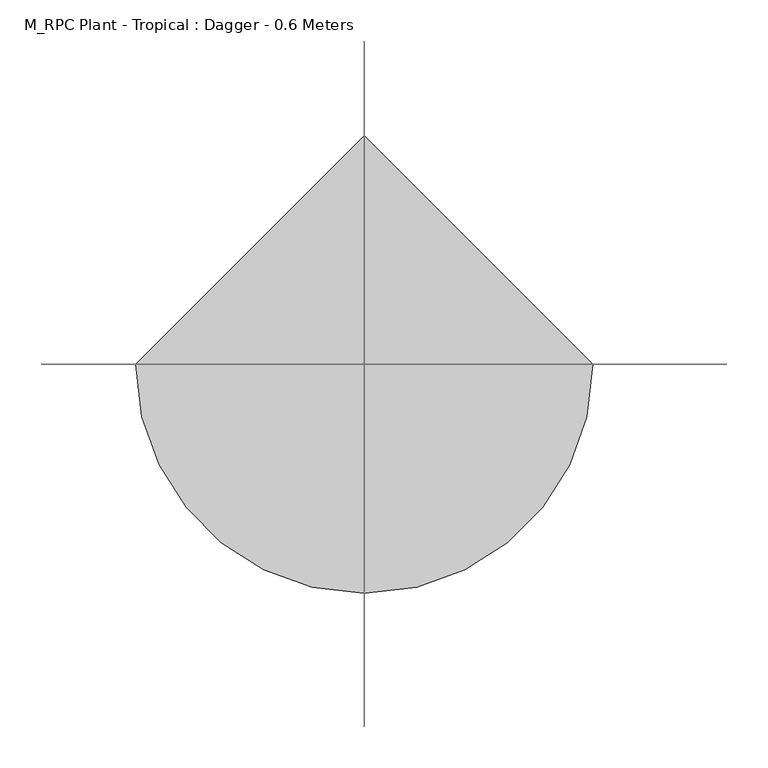
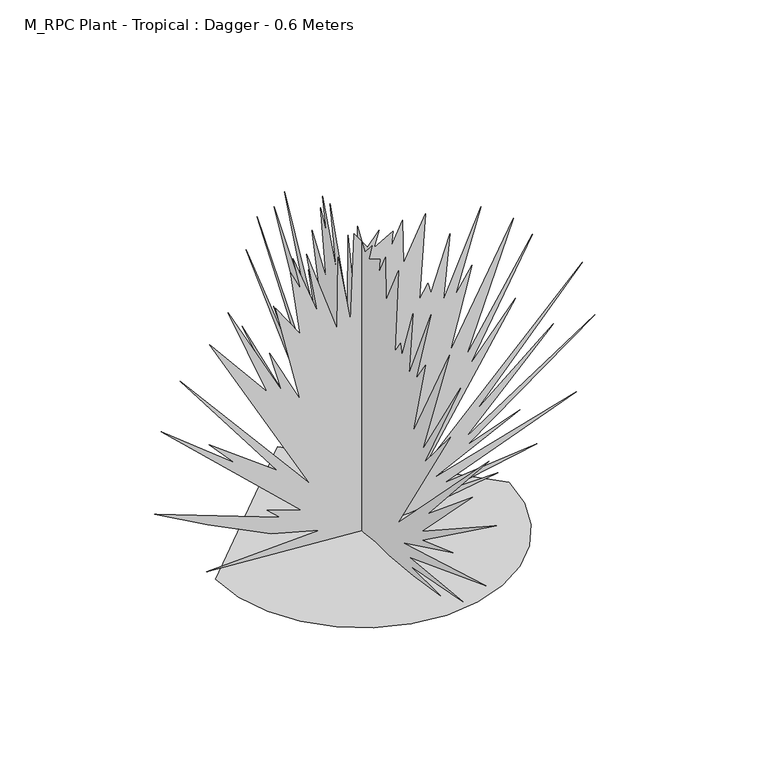
"""IFC4 building model written with IfcOpenShell, lengths in millimetres: geographic element geometry, M_RPC Plant - Tropical : Dagger - 0.6 Meters."""

from ifc_helpers import new_model, si_unit, origin, place, context, project, spatial, triangles, source, transform, mapped, element, save


def m_rpc_plant_tropical_dagger_0_6_meters_5dc34e47(model_context):
    return source(origin(), model_context, "Body", "Tessellation", [
        triangles([(0.1799897, -5.7252047, 0.0), (0.1800089, 294.2752427, 20.8333418), (0.1799966, 80.3860635, 29.1667744), (0.1800035, 172.052634, 54.1667927), (0.1800144, 292.8852294, 115.2778382), (0.1800237, 392.885321, 170.8333952), (0.1800042, 155.3861186, 81.9445621), (0.180007, 180.386137, 104.166834), (0.1800018, 115.1083446, 81.9445621), (0.1800325, 380.3853209, 331.9452544), (0.1800176, 241.4971961, 220.8334319), (0.1800237, 290.1077282, 273.610225), (0.1800103, 160.9416298, 177.7778841), (0.1800356, 344.2752794, 419.4453278), (0.1800038, 99.8305798, 130.555603), (0.1800355, 288.720222, 473.6103719), (0.1800212, 180.386137, 341.6677714), (0.1800365, 253.9977048, 525.0004037), (0.1800191, 152.608363, 334.7227738), (0.1800253, 174.8306439, 416.6678447), (0.1800152, 117.8860911, 304.1677348), (0.1800298, 163.7193854, 502.7778866), (0.1800231, 117.8860911, 436.1103353), (0.1800318, 135.9416114, 563.8904354), (0.1800283, 116.4970952, 525.0004037), (0.180033, 130.3861002, 590.2779599), (0.180023, 84.5525697, 468.0553694), (0.1800315, 105.3860819, 590.2779599), (0.1800179, 47.0527875, 420.8328521), (0.1800264, 45.663787, 563.8904354), (0.1800169, 22.052617, 427.7778497), (0.1800267, 15.1081371, 600.0004769), (0.1800231, -9.8918074, 563.8904354), (0.1800233, -32.1140259, 590.2779599), (0.180022, -22.3918427, 558.3329621), (0.1800211, -58.503047, 579.1679549), (0.1800196, -55.7252959, 551.3904353), (0.1800209, -76.5585628, 594.4454744), (0.1800157, -77.9475587, 508.3328891), (0.1800183, -119.6140924, 593.0554793), (0.1800089, -108.5030882, 425.0003303), (0.1800095, -125.1698489, 451.3903619), (0.180008, -130.725351, 430.5553328), (0.1800121, -166.8363826, 536.110445), (0.1800052, -154.3363825, 408.3328156), (0.1800106, -225.1696861, 569.4454379), (0.180004, -176.5586453, 411.1103351), (0.180005, -208.5031707, 458.3328524), (0.179998, -166.8363826, 300.0002385), (0.1800043, -286.2802365, 525.0004037), (0.1799951, -197.3919122, 281.9452177), (0.1799995, -322.3927488, 480.5553695), (0.1799934, -204.3364192, 261.1102067), (0.1799944, -290.4477329, 363.8902885), (0.1799882, -118.2253418, 87.5000733), (0.1799886, -416.8378198, 391.6678082), (0.1799871, -215.4476778, 165.277884), (0.1799856, -362.6703049, 287.5002384), (0.1799854, -196.0031525, 118.0555938), (0.1799804, -440.4478612, 277.7777214), (0.1799843, -198.7809081, 101.3890784), (0.1799804, -298.7802366, 137.5001101), (0.1799855, -134.8918572, 58.3332944), (0.179974, -405.7253077, 136.1111051), (0.1799833, -155.7253784, 41.6667836), (0.1799738, -330.7252707, 58.3332944), (0.1799822, -157.11412, 25.0000206), (0.1799763, -257.1152108, 26.3890211), (0.1799808, -168.2253785, 12.5000103), (0.1799851, -87.669567, 4.1666533), (0.1799877, -43.2252867, 4.1666533), (-277.616067, 0.0, 0.0922626), (-270.2710575, -63.6563025, 0.0922626), (-249.3550376, -122.1145939, 0.0922626), (-216.5405072, -173.6998808, 0.0922626), (-173.5032177, -216.7371703, 0.0922626), (-121.9179216, -249.5517008, 0.0922626), (-63.4596303, -270.4677206, 0.0922626), (0.1966832, -277.8127301, 0.0922626), (63.8529748, -270.4677206, 0.0922626), (122.3112661, -249.5517008, 0.0922626), (173.896544, -216.7371703, 0.0922626), (216.9338335, -173.6998808, 0.0922626), (249.7483639, -122.1145939, 0.0922626), (270.6643837, -63.6563025, 0.0922626), (278.0093933, 2.43e-05, 0.0922626), (0.1966346, 277.8127301, 0.0922626), (5.9218758, 0.016681, 0.0), (-294.0785796, 0.0166798, 20.8333418), (-80.1893913, 0.0166793, 29.1667744), (-171.8562252, 0.0166778, 54.1667927), (-292.6885663, 0.0166741, 115.2778382), (-392.6886397, 0.0166708, 170.8333952), (-155.1894555, 0.0166761, 81.9445621), (-180.1894738, 0.0166748, 104.166834), (-114.9116723, 0.0166761, 81.9445621), (-380.1886396, 0.0166612, 331.9452544), (-241.3005329, 0.0166679, 220.8334319), (-289.9110651, 0.0166647, 273.610225), (-160.7449667, 0.0166704, 177.7778841), (-344.0785981, 0.016656, 419.4453278), (-99.6339076, 0.0166732, 130.555603), (-288.5235589, 0.0166528, 473.6103719), (-180.1894738, 0.0166607, 341.6677714), (-253.8010417, 0.0166497, 525.0004037), (-152.4116999, 0.0166611, 334.7227738), (-174.6339808, 0.0166562, 416.6678447), (-117.6894188, 0.0166629, 304.1677348), (-163.5227222, 0.016651, 502.7778866), (-117.6894188, 0.016655, 436.1103353), (-135.7449392, 0.0166474, 563.8904354), (-116.300423, 0.0166497, 525.0004037), (-130.189428, 0.0166458, 590.2779599), (-84.3558975, 0.0166531, 468.0553694), (-105.1894097, 0.0166458, 590.2779599), (-46.8561152, 0.0166559, 420.8328521), (-45.4671148, 0.0166474, 563.8904354), (-21.855947, 0.0166555, 427.7778497), (-14.911491, 0.0166453, 600.0004769), (10.0885035, 0.0166474, 563.8904354), (32.3106959, 0.0166458, 590.2779599), (22.5885127, 0.0166477, 558.3329621), (58.6997192, 0.0166465, 579.1679549), (55.9219681, 0.0166481, 551.3904353), (76.755235, 0.0166456, 594.4454744), (78.1442309, 0.0166507, 508.3328891), (119.8107646, 0.0166457, 593.0554793), (108.6997604, 0.0166557, 425.0003303), (125.3665211, 0.0166541, 451.3903619), (130.9220232, 0.0166553, 430.5553328), (167.0330458, 0.0166491, 536.110445), (154.5330457, 0.0166567, 408.3328156), (225.3663493, 0.0166471, 569.4454379), (176.7553084, 0.0166565, 411.1103351), (208.6998339, 0.0166537, 458.3328524), (167.0330458, 0.0166631, 300.0002385), (286.4768997, 0.0166497, 525.0004037), (197.5885753, 0.0166642, 281.9452177), (322.5894301, 0.0166524, 480.5553695), (204.5330824, 0.0166655, 261.1102067), (290.644396, 0.0166593, 363.8902885), (118.422014, 0.0166758, 87.5000733), (417.0345011, 0.0166577, 391.6678082), (215.6443409, 0.0166712, 165.277884), (362.8669862, 0.0166639, 287.5002384), (196.1998156, 0.016674, 118.0555938), (440.6445425, 0.0166645, 277.7777214), (198.9775712, 0.016675, 101.3890784), (298.9768998, 0.0166728, 137.5001101), (135.0885294, 0.0166776, 58.3332944), (405.921989, 0.0166729, 136.1111051), (155.9220416, 0.0166785, 41.6667836), (330.9219521, 0.0166776, 58.3332944), (157.3107831, 0.0166795, 25.0000206), (257.3118739, 0.0166795, 26.3890211), (168.4220417, 0.0166803, 12.5000103), (87.8662392, 0.0166808, 4.1666533), (43.4219589, 0.0166808, 4.1666533)], [[68, 67, 69], [69, 67, 70], [64, 63, 65], [62, 61, 63], [58, 57, 59], [56, 55, 57], [57, 55, 59], [52, 51, 53], [50, 49, 51], [48, 47, 49], [46, 45, 47], [47, 45, 49], [40, 39, 41], [36, 35, 37], [34, 33, 35], [28, 27, 29], [26, 25, 27], [24, 23, 25], [22, 21, 23], [20, 19, 21], [16, 15, 17], [12, 11, 13], [10, 9, 11], [11, 9, 13], [8, 7, 9], [2, 1, 3], [66, 65, 67], [67, 65, 70], [65, 63, 70], [60, 59, 61], [61, 59, 63], [59, 55, 63], [63, 55, 70], [54, 53, 55], [53, 51, 55], [51, 49, 55], [49, 45, 55], [44, 43, 45], [45, 43, 55], [43, 42, 55], [42, 41, 55], [55, 41, 70], [41, 39, 70], [70, 39, 71], [39, 38, 71], [38, 37, 71], [37, 35, 71], [71, 35, 1], [35, 33, 1], [33, 32, 1], [18, 17, 19], [17, 15, 19], [19, 15, 21], [14, 13, 15], [13, 9, 15], [6, 5, 7], [5, 4, 7], [4, 3, 7], [7, 3, 9], [9, 3, 15], [21, 15, 23], [23, 15, 25], [25, 15, 27], [15, 3, 27], [27, 3, 29], [3, 1, 29], [29, 1, 30], [30, 1, 31], [1, 32, 31], [86, 87, 72], [85, 86, 72], [85, 72, 73], [84, 85, 73], [84, 73, 74], [84, 74, 75], [83, 84, 75], [82, 83, 75], [82, 75, 76], [82, 76, 77], [82, 77, 78], [82, 78, 79], [82, 79, 80], [82, 80, 81], [154, 155, 156], [154, 156, 157], [150, 151, 152], [148, 149, 150], [144, 145, 146], [142, 143, 144], [142, 144, 146], [138, 139, 140], [136, 137, 138], [134, 135, 136], [132, 133, 134], [132, 134, 136], [126, 127, 128], [122, 123, 124], [120, 121, 122], [114, 115, 116], [112, 113, 114], [110, 111, 112], [108, 109, 110], [106, 107, 108], [102, 103, 104], [98, 99, 100], [96, 97, 98], [96, 98, 100], [94, 95, 96], [88, 89, 90], [152, 153, 154], [152, 154, 157], [150, 152, 157], [146, 147, 148], [146, 148, 150], [142, 146, 150], [142, 150, 157], [140, 141, 142], [138, 140, 142], [136, 138, 142], [132, 136, 142], [130, 131, 132], [130, 132, 142], [129, 130, 142], [128, 129, 142], [128, 142, 157], [126, 128, 157], [126, 157, 158], [125, 126, 158], [124, 125, 158], [122, 124, 158], [122, 158, 88], [120, 122, 88], [119, 120, 88], [104, 105, 106], [102, 104, 106], [102, 106, 108], [100, 101, 102], [96, 100, 102], [92, 93, 94], [91, 92, 94], [90, 91, 94], [90, 94, 96], [90, 96, 102], [102, 108, 110], [102, 110, 112], [102, 112, 114], [90, 102, 114], [90, 114, 116], [88, 90, 116], [88, 116, 117], [88, 117, 118], [119, 88, 118]], closed=False),
    ])


if __name__ == "__main__":
    model = new_model("IFC4")
    model_context = context("Model", 3, world=origin())
    ifc_project = project(units=[si_unit("LENGTHUNIT", "METRE", prefix="MILLI")], contexts=[model_context])
    site = spatial("IfcSite", under=ifc_project)
    building = spatial("IfcBuilding", under=site)
    placement = place(None, origin())
    m_rpc_plant_tropical_dagger_0_6_meters_shape = m_rpc_plant_tropical_dagger_0_6_meters_5dc34e47(model_context)
    element("IfcGeographicElement", 1, ObjectType="M_RPC Plant - Tropical : Dagger - 0.6 Meters", at=placement, inside=building, context=model_context, shape_type="MappedRepresentation", body=[
        mapped(m_rpc_plant_tropical_dagger_0_6_meters_shape, transform((0.0, 0.0, 0.0), x_axis=(1.0, 0.0, 0.0), y_axis=(0.0, 1.0, 0.0), z_axis=(0.0, 0.0, 1.0))),
    ])
    save(model, "model.ifc")

# Revit data of these elements
# Type "M_RPC Plant - Tropical : Dagger - 0.6 Meters"
#   built-in parameter 1005198 = "{2, 15},{39, RPC-16-G3A7-NEG0-UH6H-J000-ST1L-LVER-AU},{1, 0},{1, 0},{2, 13},{1, 8},{5, Color},{1, 0},{1, 0},{3, 0.8},{3, 0.8},{3, 0.8},{1, 8},{7, BBoxMin},{1, 0},{1, 0},{1, 0},{1, 0},{1, 0},{1, 8},{7, BBoxMax},{1, 0},{1, 0},{1, 0},{1, 0},{1, 0},{2, 11},{9, RPCTypeId},{1, 0},{1, 0},{39, RPC-16-G3A7-NEG0-UH6H-J000-ST1L-LVER-AU},{1, 6},{14, RPCPlantHeight},{1, 0},{1, 0},{6, 1.9685},{2, 11},{7, keyword},{1, 0},{1, 0},{35, :RPCs:Plants [General]:Geometry:RPC},{2, 11},{8, category},{1, 0},{1, 0},{16, Plants [General]},{2, 11},{12, LocalizedUID},{1, 0},{1, 0},{6, Dagger},{2, 14},{6, Height},{1, 0},{1, 0},{6, 1.9685},{1, 2},{16, Cast Reflections},{1, 0},{1, 0},{1, 0},{1, 2},{12, Cast Shadows},{1, 0},{1, 0},{1, 1},{1, 2},{9, Lock View},{1, 0},{1, 0},{1, 0},{1, 4},{5, ViewC},{1, 0},{1, 0},{1, 0},{21, assetlibrary_base.fbx},{1, 5},"
#   built-in parameter 1005195 = "RPC-16-G3A7-NEG0-UH6H-J000-ST1L-LVER-AU"
#   Type Comments = "Dagger"
#   Height = 600 mm
#   Description = (empty or 0)
#   Default Elevation = 0
